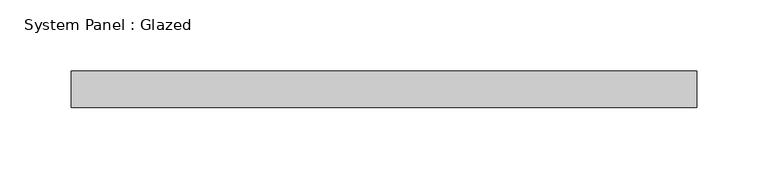
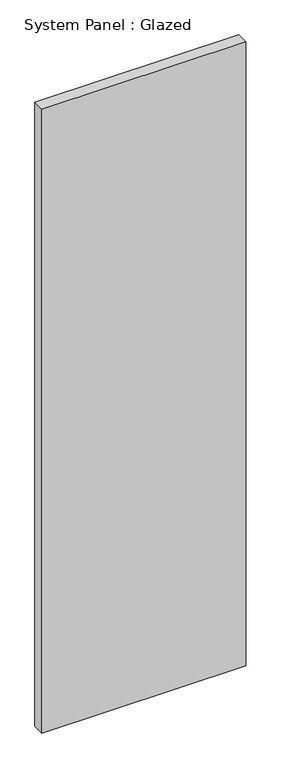
"""IFC4 building model written with IfcOpenShell, lengths in millimetres: plate geometry, System Panel : Glazed."""

from ifc_helpers import new_model, si_unit, origin, origin_with_axes, place, context, project, spatial, polyline, outline, extrude, source, transform, mapped, element, save


def system_panel_glazed_60974b7d(model_context):
    return source(origin(), model_context, "Body", "SweptSolid", [
        extrude(outline(polyline([(219.075, 19.05), (-219.075, 19.05), (-219.075, 44.45), (219.075, 44.45), (219.075, 19.05)])), origin_with_axes(), (0.0, 0.0, 1.0), 1417.4066766),
    ])


if __name__ == "__main__":
    model = new_model("IFC4")
    model_context = context("Model", 3, world=origin())
    ifc_project = project(units=[si_unit("LENGTHUNIT", "METRE", prefix="MILLI")], contexts=[model_context])
    site = spatial("IfcSite", under=ifc_project)
    building = spatial("IfcBuilding", under=site)
    placement = place(None, origin())
    system_panel_glazed_shape = system_panel_glazed_60974b7d(model_context)
    element("IfcPlate", 1, ObjectType="System Panel : Glazed", at=placement, inside=building, context=model_context, shape_type="MappedRepresentation", body=[
        mapped(system_panel_glazed_shape, transform((0.0, 0.0, 0.0), x_axis=(1.0, 0.0, 0.0), y_axis=(0.0, 1.0, 0.0), z_axis=(0.0, 0.0, 1.0))),
    ])
    save(model, "model.ifc")

# Revit data of these elements
# Type "System Panel : Glazed"
#   Construction Type Id = "GSP4R"
#   Analytic Construction = "1/8 in Pilkington single glazing"
#   Visual Light Transmittance = 0.9
#   Solar Heat Gain Coefficient = 0.86
#   Heat Transfer Coefficient (U) = 1.18115 BTU/(h·ft²·°F)
#   Define Thermal Properties by = 1
# Element 1 (IfcPlate, "System Panel : Glazed")
#   Materials on its faces: "Glass"
# Materials
#   "Glass": class "Glass", colour RGB 0 128 192, transparency 0.75, Description = "Soda Lime Glass", Cost = 0
